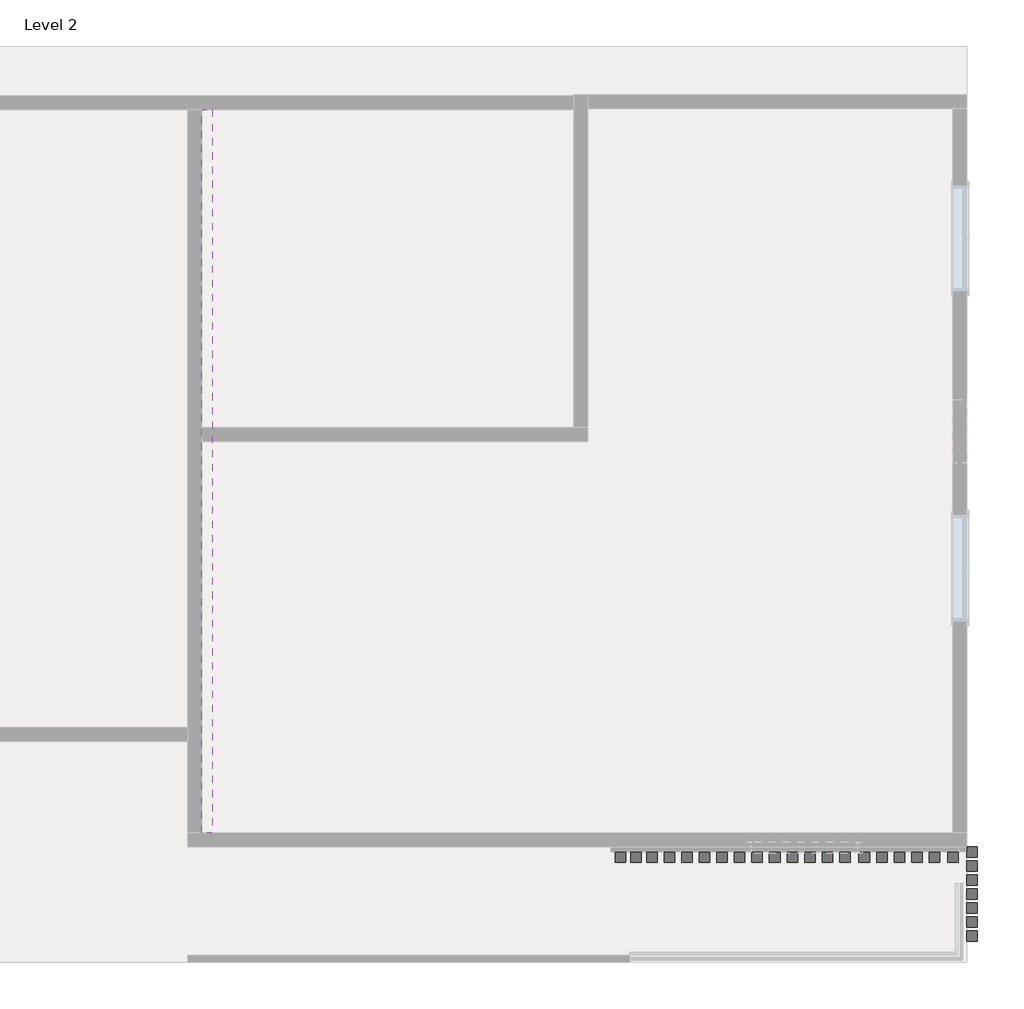
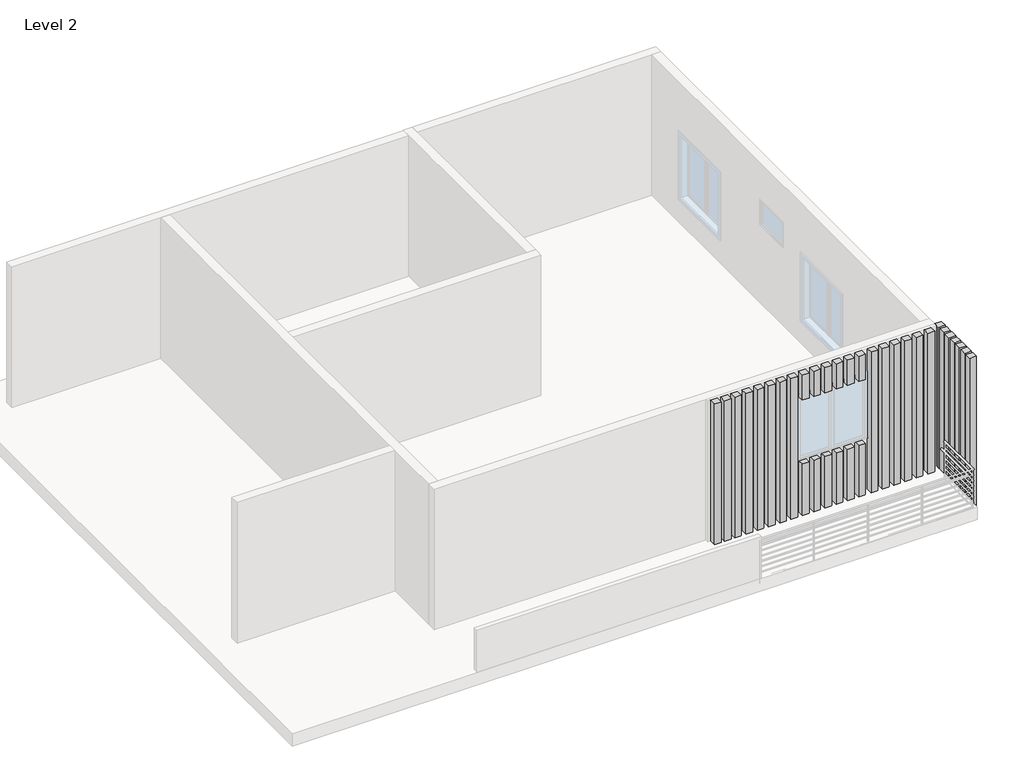
# One storey, part 2 of 2: 28 proxies.
"""IFC4 building model written with IfcOpenShell, lengths in millimetres."""

from ifc_helpers import new_model, si_unit, frame, origin, place, context, project, spatial, polyline, outline, extrude, element, save

model = new_model("IFC4")

# Units and contexts
model_context = context("Model", 3, world=origin())
ifc_project = project(units=[si_unit("LENGTHUNIT", "METRE", prefix="MILLI")], contexts=[model_context])

# Site, building, storey
site = spatial("IfcSite", under=ifc_project)
building = spatial("IfcBuilding", under=site)
storey = spatial("IfcBuildingStorey", under=building, Name="Level 2", Elevation=3657.6)

# Proxies
placement = place(None, origin())
element("IfcBuildingElementProxy", 1, Name="Cornice", ObjectType="Cornice", at=placement, inside=storey, context=model_context, shape_type="SweptSolid", body=[
    extrude(outline(polyline([(1123.5250851, -934.1518013), (1123.5250851, -1086.5518013), (971.1250851, -1086.5518013), (971.1250851, -934.1518013), (1123.5250851, -934.1518013)])), frame((0.0, 0.0, 3657.6), z_axis=(0.0, 0.0, 1.0), x_axis=(1.0, 0.0, 0.0)), (0.0, 0.0, 1.0), 3657.6),
])
element("IfcBuildingElementProxy", 2, Name="Cornice", ObjectType="Cornice", at=placement, inside=storey, context=model_context, shape_type="SweptSolid", body=[
    extrude(outline(polyline([(1352.1250851, -934.1518013), (1352.1250851, -1086.5518013), (1199.7250851, -1086.5518013), (1199.7250851, -934.1518013), (1352.1250851, -934.1518013)])), frame((0.0, 0.0, 3657.6), z_axis=(0.0, 0.0, 1.0), x_axis=(1.0, 0.0, 0.0)), (0.0, 0.0, 1.0), 3657.6),
])
element("IfcBuildingElementProxy", 3, Name="Cornice", ObjectType="Cornice", at=placement, inside=storey, context=model_context, shape_type="SweptSolid", body=[
    extrude(outline(polyline([(1580.7250851, -934.1518013), (1580.7250851, -1086.5518013), (1428.3250851, -1086.5518013), (1428.3250851, -934.1518013), (1580.7250851, -934.1518013)])), frame((0.0, 0.0, 3657.6), z_axis=(0.0, 0.0, 1.0), x_axis=(1.0, 0.0, 0.0)), (0.0, 0.0, 1.0), 3657.6),
])
element("IfcBuildingElementProxy", 4, Name="Cornice", ObjectType="Cornice", at=placement, inside=storey, context=model_context, shape_type="SweptSolid", body=[
    extrude(outline(polyline([(1834.7250851, -934.1518013), (1834.7250851, -1086.5518013), (1682.3250851, -1086.5518013), (1682.3250851, -934.1518013), (1834.7250851, -934.1518013)])), frame((0.0, 0.0, 3657.6), z_axis=(0.0, 0.0, 1.0), x_axis=(1.0, 0.0, 0.0)), (0.0, 0.0, 1.0), 3657.6),
])
element("IfcBuildingElementProxy", 5, Name="Cornice", ObjectType="Cornice", at=placement, inside=storey, context=model_context, shape_type="SweptSolid", body=[
    extrude(outline(polyline([(2088.7250851, -934.1518013), (2088.7250851, -1086.5518013), (1936.3250851, -1086.5518013), (1936.3250851, -934.1518013), (2088.7250851, -934.1518013)])), frame((0.0, 0.0, 3657.6), z_axis=(0.0, 0.0, 1.0), x_axis=(1.0, 0.0, 0.0)), (0.0, 0.0, 1.0), 3657.6),
])
element("IfcBuildingElementProxy", 6, Name="Cornice", ObjectType="Cornice", at=placement, inside=storey, context=model_context, shape_type="SweptSolid", body=[
    extrude(outline(polyline([(2342.7250851, -934.1518013), (2342.7250851, -1086.5518013), (2190.3250851, -1086.5518013), (2190.3250851, -934.1518013), (2342.7250851, -934.1518013)])), frame((0.0, 0.0, 3657.6), z_axis=(0.0, 0.0, 1.0), x_axis=(1.0, 0.0, 0.0)), (0.0, 0.0, 1.0), 3657.6),
])
element("IfcBuildingElementProxy", 7, Name="Cornice", ObjectType="Cornice", at=placement, inside=storey, context=model_context, shape_type="SweptSolid", body=[
    extrude(outline(polyline([(2596.7250851, -934.1518013), (2596.7250851, -1086.5518013), (2444.3250851, -1086.5518013), (2444.3250851, -934.1518013), (2596.7250851, -934.1518013)])), frame((0.0, 0.0, 3657.6), z_axis=(0.0, 0.0, 1.0), x_axis=(1.0, 0.0, 0.0)), (0.0, 0.0, 1.0), 3657.6),
])
element("IfcBuildingElementProxy", 8, Name="Cornice", ObjectType="Cornice", at=placement, inside=storey, context=model_context, shape_type="SweptSolid", body=[
    extrude(outline(polyline([(2850.7250851, -934.1518013), (2850.7250851, -1086.5518013), (2698.3250851, -1086.5518013), (2698.3250851, -934.1518013), (2850.7250851, -934.1518013)])), frame((0.0, 0.0, 3657.6), z_axis=(0.0, 0.0, 1.0), x_axis=(1.0, 0.0, 0.0)), (0.0, 0.0, 1.0), 3657.6),
])
element("IfcBuildingElementProxy", 9, Name="Cornice", ObjectType="Cornice", at=placement, inside=storey, context=model_context, shape_type="SweptSolid", body=[
    extrude(outline(polyline([(3104.7250851, -934.1518013), (3104.7250851, -1086.5518013), (2952.3250851, -1086.5518013), (2952.3250851, -934.1518013), (3104.7250851, -934.1518013)])), frame((0.0, 0.0, 3657.6), z_axis=(0.0, 0.0, 1.0), x_axis=(1.0, 0.0, 0.0)), (0.0, 0.0, 1.0), 1532.6723515),
    extrude(outline(polyline([(3104.7250851, -934.1518013), (3104.7250851, -1086.5518013), (2952.3250851, -1086.5518013), (2952.3250851, -934.1518013), (3104.7250851, -934.1518013)])), frame((0.0, 0.0, 6714.2723515), z_axis=(0.0, 0.0, 1.0), x_axis=(1.0, 0.0, 0.0)), (0.0, 0.0, 1.0), 600.9276485),
])
element("IfcBuildingElementProxy", 10, Name="Cornice", ObjectType="Cornice", at=placement, inside=storey, context=model_context, shape_type="SweptSolid", body=[
    extrude(outline(polyline([(3358.7250851, -934.1518013), (3358.7250851, -1086.5518013), (3206.3250851, -1086.5518013), (3206.3250851, -934.1518013), (3358.7250851, -934.1518013)])), frame((0.0, 0.0, 3657.6), z_axis=(0.0, 0.0, 1.0), x_axis=(1.0, 0.0, 0.0)), (0.0, 0.0, 1.0), 1532.6723515),
    extrude(outline(polyline([(3358.7250851, -934.1518013), (3358.7250851, -1086.5518013), (3206.3250851, -1086.5518013), (3206.3250851, -934.1518013), (3358.7250851, -934.1518013)])), frame((0.0, 0.0, 6714.2723515), z_axis=(0.0, 0.0, 1.0), x_axis=(1.0, 0.0, 0.0)), (0.0, 0.0, 1.0), 600.9276485),
])
element("IfcBuildingElementProxy", 11, Name="Cornice", ObjectType="Cornice", at=placement, inside=storey, context=model_context, shape_type="SweptSolid", body=[
    extrude(outline(polyline([(3612.7250851, -934.1518013), (3612.7250851, -1086.5518013), (3460.3250851, -1086.5518013), (3460.3250851, -934.1518013), (3612.7250851, -934.1518013)])), frame((0.0, 0.0, 3657.6), z_axis=(0.0, 0.0, 1.0), x_axis=(1.0, 0.0, 0.0)), (0.0, 0.0, 1.0), 1532.6723515),
    extrude(outline(polyline([(3612.7250851, -934.1518013), (3612.7250851, -1086.5518013), (3460.3250851, -1086.5518013), (3460.3250851, -934.1518013), (3612.7250851, -934.1518013)])), frame((0.0, 0.0, 6714.2723515), z_axis=(0.0, 0.0, 1.0), x_axis=(1.0, 0.0, 0.0)), (0.0, 0.0, 1.0), 600.9276485),
])
element("IfcBuildingElementProxy", 12, Name="Cornice", ObjectType="Cornice", at=placement, inside=storey, context=model_context, shape_type="SweptSolid", body=[
    extrude(outline(polyline([(3866.7250851, -934.1518013), (3866.7250851, -1086.5518013), (3714.3250851, -1086.5518013), (3714.3250851, -934.1518013), (3866.7250851, -934.1518013)])), frame((0.0, 0.0, 3657.6), z_axis=(0.0, 0.0, 1.0), x_axis=(1.0, 0.0, 0.0)), (0.0, 0.0, 1.0), 1532.6723515),
    extrude(outline(polyline([(3866.7250851, -934.1518013), (3866.7250851, -1086.5518013), (3714.3250851, -1086.5518013), (3714.3250851, -934.1518013), (3866.7250851, -934.1518013)])), frame((0.0, 0.0, 6714.2723515), z_axis=(0.0, 0.0, 1.0), x_axis=(1.0, 0.0, 0.0)), (0.0, 0.0, 1.0), 600.9276485),
])
element("IfcBuildingElementProxy", 13, Name="Cornice", ObjectType="Cornice", at=placement, inside=storey, context=model_context, shape_type="SweptSolid", body=[
    extrude(outline(polyline([(4120.7250851, -934.1518013), (4120.7250851, -1086.5518013), (3968.3250851, -1086.5518013), (3968.3250851, -934.1518013), (4120.7250851, -934.1518013)])), frame((0.0, 0.0, 3657.6), z_axis=(0.0, 0.0, 1.0), x_axis=(1.0, 0.0, 0.0)), (0.0, 0.0, 1.0), 1532.6723515),
    extrude(outline(polyline([(4120.7250851, -934.1518013), (4120.7250851, -1086.5518013), (3968.3250851, -1086.5518013), (3968.3250851, -934.1518013), (4120.7250851, -934.1518013)])), frame((0.0, 0.0, 6714.2723515), z_axis=(0.0, 0.0, 1.0), x_axis=(1.0, 0.0, 0.0)), (0.0, 0.0, 1.0), 600.9276485),
])
element("IfcBuildingElementProxy", 14, Name="Cornice", ObjectType="Cornice", at=placement, inside=storey, context=model_context, shape_type="SweptSolid", body=[
    extrude(outline(polyline([(4374.7250851, -934.1518013), (4374.7250851, -1086.5518013), (4222.3250851, -1086.5518013), (4222.3250851, -934.1518013), (4374.7250851, -934.1518013)])), frame((0.0, 0.0, 3657.6), z_axis=(0.0, 0.0, 1.0), x_axis=(1.0, 0.0, 0.0)), (0.0, 0.0, 1.0), 1532.6723515),
    extrude(outline(polyline([(4374.7250851, -934.1518013), (4374.7250851, -1086.5518013), (4222.3250851, -1086.5518013), (4222.3250851, -934.1518013), (4374.7250851, -934.1518013)])), frame((0.0, 0.0, 6714.2723515), z_axis=(0.0, 0.0, 1.0), x_axis=(1.0, 0.0, 0.0)), (0.0, 0.0, 1.0), 600.9276485),
])
element("IfcBuildingElementProxy", 15, Name="Cornice", ObjectType="Cornice", at=placement, inside=storey, context=model_context, shape_type="SweptSolid", body=[
    extrude(outline(polyline([(4654.1250851, -934.1518013), (4654.1250851, -1086.5518013), (4501.7250851, -1086.5518013), (4501.7250851, -934.1518013), (4654.1250851, -934.1518013)])), frame((0.0, 0.0, 3657.6), z_axis=(0.0, 0.0, 1.0), x_axis=(1.0, 0.0, 0.0)), (0.0, 0.0, 1.0), 3657.6),
])
element("IfcBuildingElementProxy", 16, Name="Cornice", ObjectType="Cornice", at=placement, inside=storey, context=model_context, shape_type="SweptSolid", body=[
    extrude(outline(polyline([(4908.1250851, -934.1518013), (4908.1250851, -1086.5518013), (4755.7250851, -1086.5518013), (4755.7250851, -934.1518013), (4908.1250851, -934.1518013)])), frame((0.0, 0.0, 3657.6), z_axis=(0.0, 0.0, 1.0), x_axis=(1.0, 0.0, 0.0)), (0.0, 0.0, 1.0), 3657.6),
])
element("IfcBuildingElementProxy", 17, Name="Cornice", ObjectType="Cornice", at=placement, inside=storey, context=model_context, shape_type="SweptSolid", body=[
    extrude(outline(polyline([(5162.1250851, -934.1518013), (5162.1250851, -1086.5518013), (5009.7250851, -1086.5518013), (5009.7250851, -934.1518013), (5162.1250851, -934.1518013)])), frame((0.0, 0.0, 3657.6), z_axis=(0.0, 0.0, 1.0), x_axis=(1.0, 0.0, 0.0)), (0.0, 0.0, 1.0), 3657.6),
])
element("IfcBuildingElementProxy", 18, Name="Cornice", ObjectType="Cornice", at=placement, inside=storey, context=model_context, shape_type="SweptSolid", body=[
    extrude(outline(polyline([(5416.1250851, -934.1518013), (5416.1250851, -1086.5518013), (5263.7250851, -1086.5518013), (5263.7250851, -934.1518013), (5416.1250851, -934.1518013)])), frame((0.0, 0.0, 3657.6), z_axis=(0.0, 0.0, 1.0), x_axis=(1.0, 0.0, 0.0)), (0.0, 0.0, 1.0), 3657.6),
])
element("IfcBuildingElementProxy", 19, Name="Cornice", ObjectType="Cornice", at=placement, inside=storey, context=model_context, shape_type="SweptSolid", body=[
    extrude(outline(polyline([(5670.1250851, -934.1518013), (5670.1250851, -1086.5518013), (5517.7250851, -1086.5518013), (5517.7250851, -934.1518013), (5670.1250851, -934.1518013)])), frame((0.0, 0.0, 3657.6), z_axis=(0.0, 0.0, 1.0), x_axis=(1.0, 0.0, 0.0)), (0.0, 0.0, 1.0), 3657.6),
])
element("IfcBuildingElementProxy", 20, Name="Cornice", ObjectType="Cornice", at=placement, inside=storey, context=model_context, shape_type="SweptSolid", body=[
    extrude(outline(polyline([(5936.8250851, -934.1518013), (5936.8250851, -1086.5518013), (5784.4250851, -1086.5518013), (5784.4250851, -934.1518013), (5936.8250851, -934.1518013)])), frame((0.0, 0.0, 3657.6), z_axis=(0.0, 0.0, 1.0), x_axis=(1.0, 0.0, 0.0)), (0.0, 0.0, 1.0), 3657.6),
])
element("IfcBuildingElementProxy", 21, Name="Cornice", ObjectType="Cornice", at=placement, inside=storey, context=model_context, shape_type="SweptSolid", body=[
    extrude(outline(polyline([(6063.8250851, -860.9451257), (6216.2250851, -860.9451257), (6216.2250851, -1013.3451257), (6063.8250851, -1013.3451257), (6063.8250851, -860.9451257)])), frame((0.0, 0.0, 3657.6), z_axis=(0.0, 0.0, 1.0), x_axis=(1.0, 0.0, 0.0)), (0.0, 0.0, 1.0), 3657.6),
])
element("IfcBuildingElementProxy", 22, Name="Cornice", ObjectType="Cornice", at=placement, inside=storey, context=model_context, shape_type="SweptSolid", body=[
    extrude(outline(polyline([(6063.8250851, -1064.1451257), (6216.2250851, -1064.1451257), (6216.2250851, -1216.5451257), (6063.8250851, -1216.5451257), (6063.8250851, -1064.1451257)])), frame((0.0, 0.0, 3657.6), z_axis=(0.0, 0.0, 1.0), x_axis=(1.0, 0.0, 0.0)), (0.0, 0.0, 1.0), 3657.6),
])
element("IfcBuildingElementProxy", 23, Name="Cornice", ObjectType="Cornice", at=placement, inside=storey, context=model_context, shape_type="SweptSolid", body=[
    extrude(outline(polyline([(6063.8250851, -1267.3451257), (6216.2250851, -1267.3451257), (6216.2250851, -1419.7451257), (6063.8250851, -1419.7451257), (6063.8250851, -1267.3451257)])), frame((0.0, 0.0, 3657.6), z_axis=(0.0, 0.0, 1.0), x_axis=(1.0, 0.0, 0.0)), (0.0, 0.0, 1.0), 3657.6),
])
element("IfcBuildingElementProxy", 24, Name="Cornice", ObjectType="Cornice", at=placement, inside=storey, context=model_context, shape_type="SweptSolid", body=[
    extrude(outline(polyline([(6063.8250851, -1470.5451257), (6216.2250851, -1470.5451257), (6216.2250851, -1622.9451257), (6063.8250851, -1622.9451257), (6063.8250851, -1470.5451257)])), frame((0.0, 0.0, 3657.6), z_axis=(0.0, 0.0, 1.0), x_axis=(1.0, 0.0, 0.0)), (0.0, 0.0, 1.0), 3657.6),
])
element("IfcBuildingElementProxy", 25, Name="Cornice", ObjectType="Cornice", at=placement, inside=storey, context=model_context, shape_type="SweptSolid", body=[
    extrude(outline(polyline([(6063.8250851, -1673.7451257), (6216.2250851, -1673.7451257), (6216.2250851, -1826.1451257), (6063.8250851, -1826.1451257), (6063.8250851, -1673.7451257)])), frame((0.0, 0.0, 3657.6), z_axis=(0.0, 0.0, 1.0), x_axis=(1.0, 0.0, 0.0)), (0.0, 0.0, 1.0), 3657.6),
])
element("IfcBuildingElementProxy", 26, Name="Cornice", ObjectType="Cornice", at=placement, inside=storey, context=model_context, shape_type="SweptSolid", body=[
    extrude(outline(polyline([(6063.8250851, -1876.9451257), (6216.2250851, -1876.9451257), (6216.2250851, -2029.3451257), (6063.8250851, -2029.3451257), (6063.8250851, -1876.9451257)])), frame((0.0, 0.0, 3657.6), z_axis=(0.0, 0.0, 1.0), x_axis=(1.0, 0.0, 0.0)), (0.0, 0.0, 1.0), 3657.6),
])
element("IfcBuildingElementProxy", 27, Name="Cornice", ObjectType="Cornice", at=placement, inside=storey, context=model_context, shape_type="SweptSolid", body=[
    extrude(outline(polyline([(6063.8250851, -2080.1451257), (6216.2250851, -2080.1451257), (6216.2250851, -2232.5451257), (6063.8250851, -2232.5451257), (6063.8250851, -2080.1451257)])), frame((0.0, 0.0, 3657.6), z_axis=(0.0, 0.0, 1.0), x_axis=(1.0, 0.0, 0.0)), (0.0, 0.0, 1.0), 3657.6),
])
element("IfcBuildingElementProxy", 28, Name="Cornice", ObjectType="Cornice", at=placement, inside=storey, context=model_context, shape_type="SweptSolid", body=[
    extrude(outline(polyline([(6063.8250851, 4415.9048743), (6216.2250851, 4415.9048743), (6216.2250851, 4390.5048743), (6063.8250851, 4390.5048743), (6063.8250851, 4415.9048743)])), frame((0.0, 0.0, 6096.0), z_axis=(0.0, 0.0, 1.0), x_axis=(1.0, 0.0, 0.0)), (0.0, 0.0, 1.0), 152.4),
    extrude(outline(polyline([(6063.8250851, 4415.9048743), (6216.2250851, 4415.9048743), (6216.2250851, 1952.1048743), (6063.8250851, 1952.1048743), (6063.8250851, 4415.9048743)])), frame((0.0, 0.0, 6096.0), z_axis=(0.0, 0.0, 1.0), x_axis=(1.0, 0.0, 0.0)), (0.0, 0.0, 1.0), 152.4),
    extrude(outline(polyline([(-4858.1749149, -657.7451257), (-5010.5749149, -657.7451257), (-5010.5749149, 9807.0548743), (-4858.1749149, 9807.0548743), (-4858.1749149, -657.7451257)])), frame((0.0, 0.0, 6096.0), z_axis=(0.0, 0.0, 1.0), x_axis=(1.0, 0.0, 0.0)), (0.0, 0.0, 1.0), 152.4),
])

save(model, "model.ifc")

# Revit data of these elements
# Elements 1, 2, 3, 4, 5, 6, 7, 8, 9, 10, 11, 12, 13, 14, 15, 16, 17, 18, 19, 20, 21, 22, 23, 24, 25, 26, 27, 28 (IfcBuildingElementProxy, "Cornice")
#   Phase Created = New Construction
#   Materials on its faces: "Default Wall"
# Materials
#   "Default Wall": colour RGB 128 128 128, transparency 0
